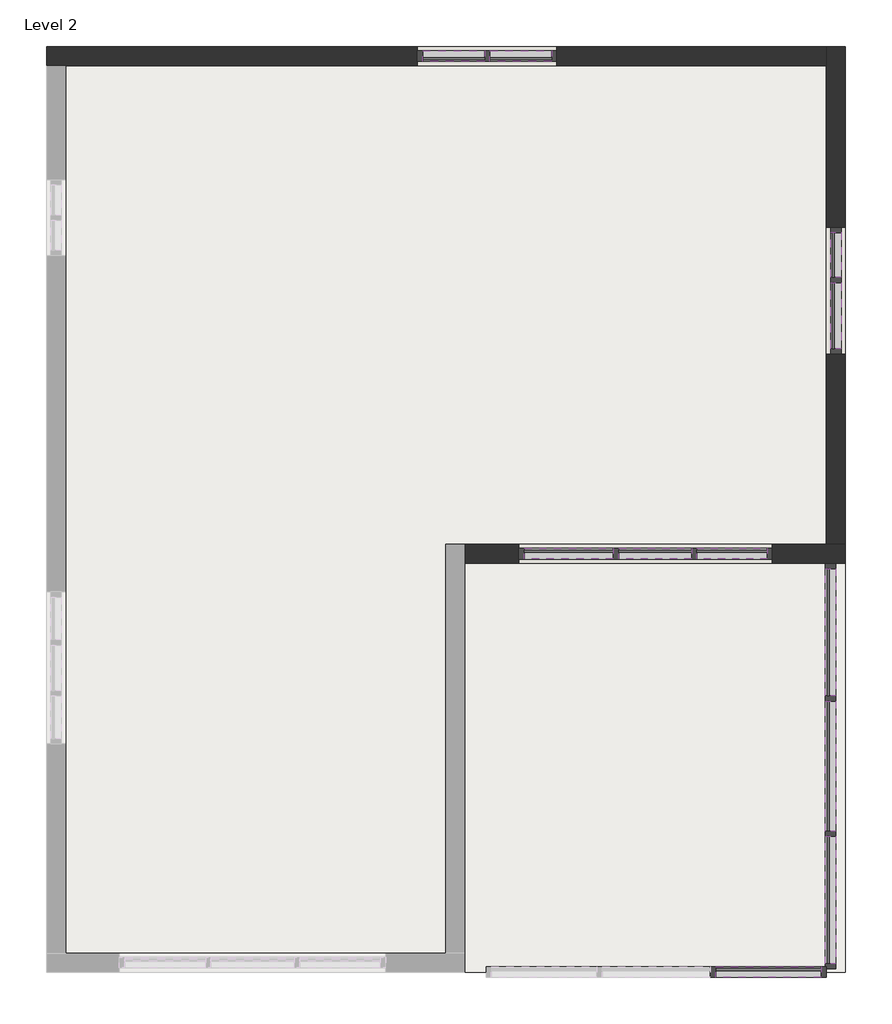
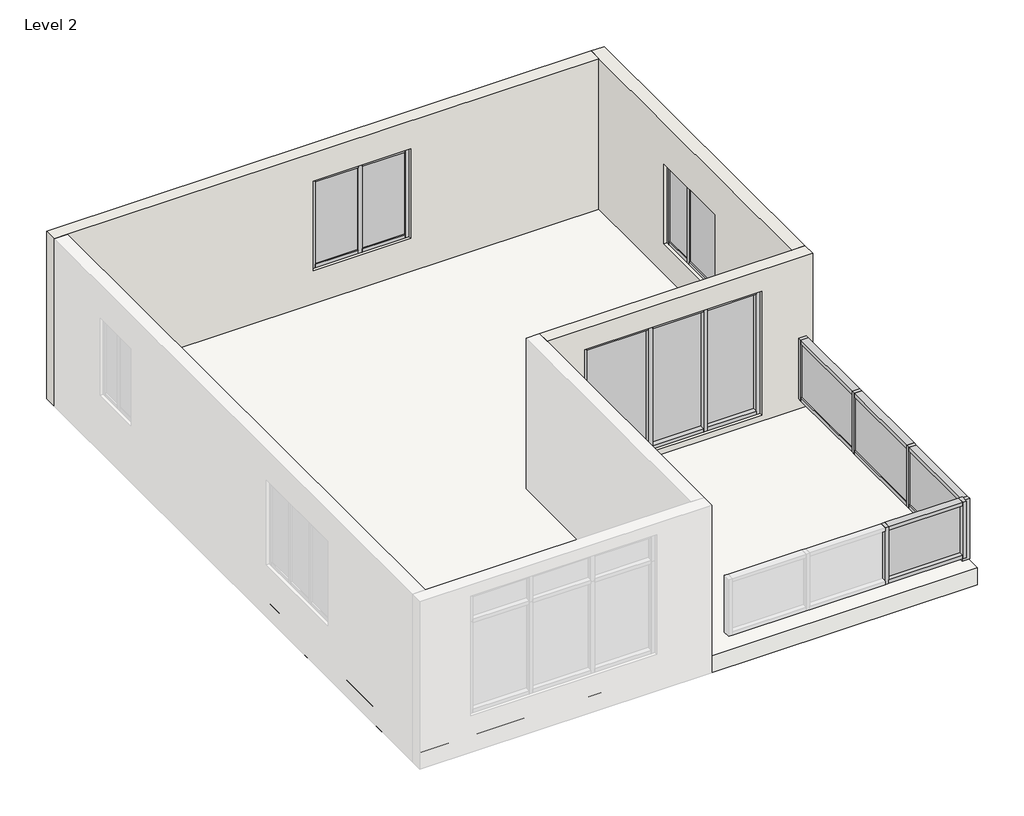
# One storey, part 2 of 2: 38 members, 11 plates, 3 walls, 1 roof.
"""IFC4 building model written with IfcOpenShell, lengths in millimetres."""

from ifc_helpers import new_model, si_unit, frame, origin, place, context, project, spatial, polyline, outline, extrude, faceted_brep, transform, mapped, element, save
from components import member_81de2198, member_99b0d556, member_4d6ef9b1, member_3974447c, member_c3d994c2, member_091e92f8, member_eb359e9e, member_20160837, member_02f15020, member_8e1b9e66, member_e29be78d, member_3eefc08a, member_e90b2f09, member_13dc6413, member_ee8fd4dd, member_c59792e9, member_3a0a7659, member_1a0dfb12, member_62f62403, system_panel_glazed_a9a9195b, system_panel_glazed_303585a9, system_panel_glazed_dbec328f, system_panel_glazed_6a79ef8b, system_panel_glazed_b7516aa2, system_panel_glazed_3160786d, system_panel_glazed_8fb7f6e3, system_panel_glazed_63ee4140, system_panel_glazed_1c093cbc

model = new_model("IFC4")

# Units and contexts
model_context = context("Model", 3, world=origin())
ifc_project = project(units=[si_unit("LENGTHUNIT", "METRE", prefix="MILLI")], contexts=[model_context])

# Site, building, storey
site = spatial("IfcSite", under=ifc_project)
building = spatial("IfcBuilding", under=site)
storey = spatial("IfcBuildingStorey", under=building, Name="Level 2", Elevation=3048.0)

# Members
placement = place(None, origin())
member_shape = member_81de2198(model_context)
element("IfcMember", 1, ObjectType="Rectangular Mullion : 2.5\" x 5\" rectangular", at=placement, inside=storey, context=model_context, shape_type="MappedRepresentation", body=[
    mapped(member_shape, transform((-8098.3518575, -6804.4878384, 3902.8712854), x_axis=(0.0, 0.0, -1.0), y_axis=(1.0, 0.0, 0.0), z_axis=(0.0, -1.0, 0.0))),
])
element("IfcMember", 2, ObjectType="Rectangular Mullion : 2.5\" x 5\" rectangular", at=placement, inside=storey, context=model_context, shape_type="MappedRepresentation", body=[
    mapped(member_shape, transform((-8098.3518575, -6264.7378384, 5354.7619868), x_axis=(0.0, 0.0, 1.0), y_axis=(1.0, 0.0, 0.0), z_axis=(0.0, 1.0, 0.0))),
])
member_2_shape = member_99b0d556(model_context)
element("IfcMember", 3, ObjectType="Rectangular Mullion : 2.5\" x 5\" rectangular", at=placement, inside=storey, context=model_context, shape_type="MappedRepresentation", body=[
    mapped(member_2_shape, transform((-10708.2018575, -10125.5378384, 3460.4214945), x_axis=(0.0, 0.0, -1.0), y_axis=(0.0, -1.0, 0.0), z_axis=(-1.0, 0.0, 0.0))),
])
member_3_shape = member_4d6ef9b1(model_context)
element("IfcMember", 4, ObjectType="Rectangular Mullion : 2.5\" x 5\" rectangular", at=placement, inside=storey, context=model_context, shape_type="MappedRepresentation", body=[
    mapped(member_3_shape, transform((-11844.8518575, -10125.5378384, 3460.4214945), x_axis=(0.0, 0.0, -1.0), y_axis=(0.0, -1.0, 0.0), z_axis=(-1.0, 0.0, 0.0))),
])
member_4_shape = member_3974447c(model_context)
element("IfcMember", 5, ObjectType="Rectangular Mullion : 2.5\" x 5\" rectangular", at=placement, inside=storey, context=model_context, shape_type="MappedRepresentation", body=[
    mapped(member_4_shape, transform((-9800.1518575, -10125.5378384, 3460.4214945), x_axis=(1.0, 0.0, 0.0), y_axis=(0.0, -1.0, 0.0), z_axis=(0.0, 0.0, -1.0))),
])
element("IfcMember", 6, ObjectType="Rectangular Mullion : 2.5\" x 5\" rectangular", at=placement, inside=storey, context=model_context, shape_type="MappedRepresentation", body=[
    mapped(member_4_shape, transform((-10739.9518575, -10125.5378384, 3460.4214945), x_axis=(1.0, 0.0, 0.0), y_axis=(0.0, -1.0, 0.0), z_axis=(0.0, 0.0, -1.0))),
])
element("IfcMember", 7, ObjectType="Rectangular Mullion : 2.5\" x 5\" rectangular", at=placement, inside=storey, context=model_context, shape_type="MappedRepresentation", body=[
    mapped(member_2_shape, transform((-9831.9018575, -10125.5378384, 5714.786093), x_axis=(0.0, 0.0, 1.0), y_axis=(0.0, -1.0, 0.0), z_axis=(1.0, 0.0, 0.0))),
])
element("IfcMember", 8, ObjectType="Rectangular Mullion : 2.5\" x 5\" rectangular", at=placement, inside=storey, context=model_context, shape_type="MappedRepresentation", body=[
    mapped(member_3_shape, transform((-10771.7018575, -10125.5378384, 5714.786093), x_axis=(0.0, 0.0, 1.0), y_axis=(0.0, -1.0, 0.0), z_axis=(1.0, 0.0, 0.0))),
])
member_5_shape = member_c3d994c2(model_context)
element("IfcMember", 9, ObjectType="Rectangular Mullion : 2.5\" x 5\" rectangular", at=placement, inside=storey, context=model_context, shape_type="MappedRepresentation", body=[
    mapped(member_5_shape, transform((-11908.3518575, -10125.5378384, 5714.786093), x_axis=(-1.0, 0.0, 0.0), y_axis=(0.0, -1.0, 0.0), z_axis=(0.0, 0.0, 1.0))),
])
member_6_shape = member_091e92f8(model_context)
element("IfcMember", 10, ObjectType="Rectangular Mullion : 2.5\" x 5\" rectangular", at=placement, inside=storey, context=model_context, shape_type="MappedRepresentation", body=[
    mapped(member_6_shape, transform((-9768.4018575, -10125.5378384, 3460.4214945), x_axis=(0.0, 0.0, -1.0), y_axis=(0.0, -1.0, 0.0), z_axis=(-1.0, 0.0, 0.0))),
])
element("IfcMember", 11, ObjectType="Rectangular Mullion : 2.5\" x 5\" rectangular", at=placement, inside=storey, context=model_context, shape_type="MappedRepresentation", body=[
    mapped(member_6_shape, transform((-8923.8518575, -10125.5378384, 5714.786093), x_axis=(0.0, 0.0, 1.0), y_axis=(0.0, -1.0, 0.0), z_axis=(1.0, 0.0, 0.0))),
])
element("IfcMember", 12, ObjectType="Rectangular Mullion : 2.5\" x 5\" rectangular", at=placement, inside=storey, context=model_context, shape_type="MappedRepresentation", body=[
    mapped(member_5_shape, transform((-8860.3518575, -10125.5378384, 3460.4214945), x_axis=(1.0, 0.0, 0.0), y_axis=(0.0, -1.0, 0.0), z_axis=(0.0, 0.0, -1.0))),
])
member_7_shape = member_eb359e9e(model_context)
element("IfcMember", 13, ObjectType="Rectangular Mullion : 2.5\" x 5\" rectangular", at=placement, inside=storey, context=model_context, shape_type="MappedRepresentation", body=[
    mapped(member_7_shape, transform((-8276.1518575, -15154.7378384, 4689.3272807), x_axis=(0.0, 0.0, 1.0), y_axis=(0.0, -1.0, 0.0), z_axis=(1.0, 0.0, 0.0))),
])
element("IfcMember", 14, ObjectType="Rectangular Mullion : 2.5\" x 5\" rectangular", at=placement, inside=storey, context=model_context, shape_type="MappedRepresentation", body=[
    mapped(member_7_shape, transform((-9544.0351909, -15154.7378384, 3657.6), x_axis=(0.0, 0.0, -1.0), y_axis=(0.0, -1.0, 0.0), z_axis=(-1.0, 0.0, 0.0))),
])
member_8_shape = member_20160837(model_context)
element("IfcMember", 15, ObjectType="Rectangular Mullion : 2.5\" x 5\" rectangular", at=placement, inside=storey, context=model_context, shape_type="MappedRepresentation", body=[
    mapped(member_8_shape, transform((-9575.7851909, -15154.7378384, 3657.6), x_axis=(1.0, 0.0, 0.0), y_axis=(0.0, -1.0, 0.0), z_axis=(0.0, 0.0, -1.0))),
])
member_9_shape = member_02f15020(model_context)
element("IfcMember", 16, ObjectType="Rectangular Mullion : 2.5\" x 5\" rectangular", at=placement, inside=storey, context=model_context, shape_type="MappedRepresentation", body=[
    mapped(member_9_shape, transform((-8212.6518575, -15154.7378384, 3657.6), x_axis=(1.0, 0.0, 0.0), y_axis=(0.0, -1.0, 0.0), z_axis=(0.0, 0.0, -1.0))),
])
member_10_shape = member_8e1b9e66(model_context)
element("IfcMember", 17, ObjectType="Rectangular Mullion : 2.5\" x 5\" rectangular", at=placement, inside=storey, context=model_context, shape_type="MappedRepresentation", body=[
    mapped(member_10_shape, transform((-8160.2387627, -13522.2465167, 4639.9432926), x_axis=(0.0, 0.0, 1.0), y_axis=(1.0, 0.0, 0.0), z_axis=(0.0, 1.0, 0.0))),
])
element("IfcMember", 18, ObjectType="Rectangular Mullion : 2.5\" x 5\" rectangular", at=placement, inside=storey, context=model_context, shape_type="MappedRepresentation", body=[
    mapped(member_10_shape, transform((-8160.2387627, -10303.3378384, 4639.9432926), x_axis=(0.0, 0.0, 1.0), y_axis=(1.0, 0.0, 0.0), z_axis=(0.0, 1.0, 0.0))),
])
member_11_shape = member_e29be78d(model_context)
element("IfcMember", 19, ObjectType="Rectangular Mullion : 2.5\" x 5\" rectangular", at=placement, inside=storey, context=model_context, shape_type="MappedRepresentation", body=[
    mapped(member_11_shape, transform((-8160.2387627, -11896.9171776, 4639.9432926), x_axis=(0.0, 0.0, 1.0), y_axis=(1.0, 0.0, 0.0), z_axis=(0.0, 1.0, 0.0))),
])
member_12_shape = member_3eefc08a(model_context)
element("IfcMember", 20, ObjectType="Rectangular Mullion : 2.5\" x 5\" rectangular", at=placement, inside=storey, context=model_context, shape_type="MappedRepresentation", body=[
    mapped(member_12_shape, transform((-8160.2387627, -13490.4965167, 3533.6625279), x_axis=(0.0, 1.0, 0.0), y_axis=(1.0, 0.0, 0.0), z_axis=(0.0, 0.0, -1.0))),
])
element("IfcMember", 21, ObjectType="Rectangular Mullion : 2.5\" x 5\" rectangular", at=placement, inside=storey, context=model_context, shape_type="MappedRepresentation", body=[
    mapped(member_12_shape, transform((-8160.2387627, -11865.1671776, 3533.6625279), x_axis=(0.0, 1.0, 0.0), y_axis=(1.0, 0.0, 0.0), z_axis=(0.0, 0.0, -1.0))),
])
element("IfcMember", 22, ObjectType="Rectangular Mullion : 2.5\" x 5\" rectangular", at=placement, inside=storey, context=model_context, shape_type="MappedRepresentation", body=[
    mapped(member_10_shape, transform((-8160.2387627, -11833.4171776, 3533.6625279), x_axis=(0.0, 0.0, -1.0), y_axis=(1.0, 0.0, 0.0), z_axis=(0.0, -1.0, 0.0))),
])
element("IfcMember", 23, ObjectType="Rectangular Mullion : 2.5\" x 5\" rectangular", at=placement, inside=storey, context=model_context, shape_type="MappedRepresentation", body=[
    mapped(member_10_shape, transform((-8160.2387627, -15052.3258559, 3533.6625279), x_axis=(0.0, 0.0, -1.0), y_axis=(1.0, 0.0, 0.0), z_axis=(0.0, -1.0, 0.0))),
])
element("IfcMember", 24, ObjectType="Rectangular Mullion : 2.5\" x 5\" rectangular", at=placement, inside=storey, context=model_context, shape_type="MappedRepresentation", body=[
    mapped(member_11_shape, transform((-8160.2387627, -13458.7465167, 3533.6625279), x_axis=(0.0, 0.0, -1.0), y_axis=(1.0, 0.0, 0.0), z_axis=(0.0, -1.0, 0.0))),
])
member_13_shape = member_e90b2f09(model_context)
element("IfcMember", 25, ObjectType="Rectangular Mullion : 2.5\" x 5\" rectangular", at=placement, inside=storey, context=model_context, shape_type="MappedRepresentation", body=[
    mapped(member_13_shape, transform((-8160.2387627, -15115.8258559, 4639.9432926), x_axis=(0.0, -1.0, 0.0), y_axis=(1.0, 0.0, 0.0), z_axis=(0.0, 0.0, 1.0))),
])
element("IfcMember", 26, ObjectType="Rectangular Mullion : 2.5\" x 5\" rectangular", at=placement, inside=storey, context=model_context, shape_type="MappedRepresentation", body=[
    mapped(member_13_shape, transform((-8160.2387627, -10239.8378384, 3533.6625279), x_axis=(0.0, 1.0, 0.0), y_axis=(1.0, 0.0, 0.0), z_axis=(0.0, 0.0, -1.0))),
])
member_14_shape = member_13dc6413(model_context)
element("IfcMember", 27, ObjectType="Rectangular Mullion : 2.5\" x 5\" rectangular", at=placement, inside=storey, context=model_context, shape_type="MappedRepresentation", body=[
    mapped(member_14_shape, transform((-8098.3518575, -6867.9878384, 5354.7619868), x_axis=(0.0, 0.0, 1.0), y_axis=(1.0, 0.0, 0.0), z_axis=(0.0, 1.0, 0.0))),
])
member_15_shape = member_ee8fd4dd(model_context)
element("IfcMember", 28, ObjectType="Rectangular Mullion : 2.5\" x 5\" rectangular", at=placement, inside=storey, context=model_context, shape_type="MappedRepresentation", body=[
    mapped(member_15_shape, transform((-8098.3518575, -6836.2378384, 3902.8712854), x_axis=(0.0, 1.0, 0.0), y_axis=(1.0, 0.0, 0.0), z_axis=(0.0, 0.0, -1.0))),
])
element("IfcMember", 29, ObjectType="Rectangular Mullion : 2.5\" x 5\" rectangular", at=placement, inside=storey, context=model_context, shape_type="MappedRepresentation", body=[
    mapped(member_14_shape, transform((-8098.3518575, -7661.7378384, 3902.8712854), x_axis=(0.0, 0.0, -1.0), y_axis=(1.0, 0.0, 0.0), z_axis=(0.0, -1.0, 0.0))),
])
member_16_shape = member_c59792e9(model_context)
element("IfcMember", 30, ObjectType="Rectangular Mullion : 2.5\" x 5\" rectangular", at=placement, inside=storey, context=model_context, shape_type="MappedRepresentation", body=[
    mapped(member_16_shape, transform((-8098.3518575, -6201.2378384, 3902.8712854), x_axis=(0.0, 1.0, 0.0), y_axis=(1.0, 0.0, 0.0), z_axis=(0.0, 0.0, -1.0))),
])
element("IfcMember", 31, ObjectType="Rectangular Mullion : 2.5\" x 5\" rectangular", at=placement, inside=storey, context=model_context, shape_type="MappedRepresentation", body=[
    mapped(member_16_shape, transform((-8098.3518575, -7725.2378384, 5354.7619868), x_axis=(0.0, -1.0, 0.0), y_axis=(1.0, 0.0, 0.0), z_axis=(0.0, 0.0, 1.0))),
])
member_17_shape = member_3a0a7659(model_context)
element("IfcMember", 32, ObjectType="Rectangular Mullion : 2.5\" x 5\" rectangular", at=placement, inside=storey, context=model_context, shape_type="MappedRepresentation", body=[
    mapped(member_17_shape, transform((-12257.6018575, -4143.8378384, 5584.2385429), x_axis=(0.0, 0.0, 1.0), y_axis=(0.0, 1.0, 0.0), z_axis=(-1.0, 0.0, 0.0))),
])
element("IfcMember", 33, ObjectType="Rectangular Mullion : 2.5\" x 5\" rectangular", at=placement, inside=storey, context=model_context, shape_type="MappedRepresentation", body=[
    mapped(member_17_shape, transform((-13064.0518575, -4143.8378384, 5584.2385429), x_axis=(0.0, 0.0, 1.0), y_axis=(0.0, 1.0, 0.0), z_axis=(-1.0, 0.0, 0.0))),
])
member_18_shape = member_1a0dfb12(model_context)
element("IfcMember", 34, ObjectType="Rectangular Mullion : 2.5\" x 5\" rectangular", at=placement, inside=storey, context=model_context, shape_type="MappedRepresentation", body=[
    mapped(member_18_shape, transform((-12289.3518575, -4143.8378384, 3955.4729812), x_axis=(-1.0, 0.0, 0.0), y_axis=(0.0, 1.0, 0.0), z_axis=(0.0, 0.0, -1.0))),
])
element("IfcMember", 35, ObjectType="Rectangular Mullion : 2.5\" x 5\" rectangular", at=placement, inside=storey, context=model_context, shape_type="MappedRepresentation", body=[
    mapped(member_17_shape, transform((-12321.1018575, -4143.8378384, 3955.4729812), x_axis=(0.0, 0.0, -1.0), y_axis=(0.0, 1.0, 0.0), z_axis=(1.0, 0.0, 0.0))),
])
element("IfcMember", 36, ObjectType="Rectangular Mullion : 2.5\" x 5\" rectangular", at=placement, inside=storey, context=model_context, shape_type="MappedRepresentation", body=[
    mapped(member_17_shape, transform((-11514.6518575, -4143.8378384, 3955.4729812), x_axis=(0.0, 0.0, -1.0), y_axis=(0.0, 1.0, 0.0), z_axis=(1.0, 0.0, 0.0))),
])
member_19_shape = member_62f62403(model_context)
element("IfcMember", 37, ObjectType="Rectangular Mullion : 2.5\" x 5\" rectangular", at=placement, inside=storey, context=model_context, shape_type="MappedRepresentation", body=[
    mapped(member_19_shape, transform((-13127.5518575, -4143.8378384, 3955.4729812), x_axis=(-1.0, 0.0, 0.0), y_axis=(0.0, 1.0, 0.0), z_axis=(0.0, 0.0, -1.0))),
])
element("IfcMember", 38, ObjectType="Rectangular Mullion : 2.5\" x 5\" rectangular", at=placement, inside=storey, context=model_context, shape_type="MappedRepresentation", body=[
    mapped(member_19_shape, transform((-11451.1518575, -4143.8378384, 5584.2385429), x_axis=(1.0, 0.0, 0.0), y_axis=(0.0, 1.0, 0.0), z_axis=(0.0, 0.0, 1.0))),
])

# Plates
system_panel_glazed_shape = system_panel_glazed_a9a9195b(model_context)
element("IfcPlate", 39, ObjectType="System Panel : Glazed", at=placement, inside=storey, context=model_context, shape_type="MappedRepresentation", body=[
    mapped(system_panel_glazed_shape, transform((-11308.2768575, -10125.5378384, 3523.9214945), x_axis=(1.0, 0.0, 0.0), y_axis=(0.0, 1.0, 0.0), z_axis=(0.0, 0.0, 1.0))),
])
system_panel_glazed_2_shape = system_panel_glazed_303585a9(model_context)
element("IfcPlate", 40, ObjectType="System Panel : Glazed", at=placement, inside=storey, context=model_context, shape_type="MappedRepresentation", body=[
    mapped(system_panel_glazed_2_shape, transform((-10270.0518575, -10125.5378384, 3523.9214945), x_axis=(1.0, 0.0, 0.0), y_axis=(0.0, 1.0, 0.0), z_axis=(0.0, 0.0, 1.0))),
])
system_panel_glazed_3_shape = system_panel_glazed_dbec328f(model_context)
element("IfcPlate", 41, ObjectType="System Panel : Glazed", at=placement, inside=storey, context=model_context, shape_type="MappedRepresentation", body=[
    mapped(system_panel_glazed_3_shape, transform((-9346.1268575, -10125.5378384, 3523.9214945), x_axis=(1.0, 0.0, 0.0), y_axis=(0.0, 1.0, 0.0), z_axis=(0.0, 0.0, 1.0))),
])
system_panel_glazed_4_shape = system_panel_glazed_6a79ef8b(model_context)
element("IfcPlate", 42, ObjectType="System Panel : Glazed", at=placement, inside=storey, context=model_context, shape_type="MappedRepresentation", body=[
    mapped(system_panel_glazed_4_shape, transform((-8910.0935242, -15154.7378384, 3721.1), x_axis=(1.0, 0.0, 0.0), y_axis=(0.0, 1.0, 0.0), z_axis=(0.0, 0.0, 1.0))),
])
system_panel_glazed_5_shape = system_panel_glazed_b7516aa2(model_context)
element("IfcPlate", 43, ObjectType="System Panel : Glazed", at=placement, inside=storey, context=model_context, shape_type="MappedRepresentation", body=[
    mapped(system_panel_glazed_5_shape, transform((-8160.2387627, -14287.2861863, 3597.1625279), x_axis=(0.0, 1.0, 0.0), y_axis=(-1.0, 0.0, 0.0), z_axis=(0.0, 0.0, 1.0))),
])
element("IfcPlate", 44, ObjectType="System Panel : Glazed", at=placement, inside=storey, context=model_context, shape_type="MappedRepresentation", body=[
    mapped(system_panel_glazed_5_shape, transform((-8160.2387627, -11068.377508, 3597.1625279), x_axis=(0.0, 1.0, 0.0), y_axis=(-1.0, 0.0, 0.0), z_axis=(0.0, 0.0, 1.0))),
])
system_panel_glazed_6_shape = system_panel_glazed_3160786d(model_context)
element("IfcPlate", 45, ObjectType="System Panel : Glazed", at=placement, inside=storey, context=model_context, shape_type="MappedRepresentation", body=[
    mapped(system_panel_glazed_6_shape, transform((-8160.2387627, -12677.8318471, 3597.1625279), x_axis=(0.0, 1.0, 0.0), y_axis=(-1.0, 0.0, 0.0), z_axis=(0.0, 0.0, 1.0))),
])
system_panel_glazed_7_shape = system_panel_glazed_8fb7f6e3(model_context)
element("IfcPlate", 46, ObjectType="System Panel : Glazed", at=placement, inside=storey, context=model_context, shape_type="MappedRepresentation", body=[
    mapped(system_panel_glazed_7_shape, transform((-8098.3518575, -7264.8628384, 3966.3712854), x_axis=(0.0, 1.0, 0.0), y_axis=(-1.0, 0.0, 0.0), z_axis=(0.0, 0.0, 1.0))),
])
system_panel_glazed_8_shape = system_panel_glazed_63ee4140(model_context)
element("IfcPlate", 47, ObjectType="System Panel : Glazed", at=placement, inside=storey, context=model_context, shape_type="MappedRepresentation", body=[
    mapped(system_panel_glazed_8_shape, transform((-8098.3518575, -6534.6128384, 3966.3712854), x_axis=(0.0, 1.0, 0.0), y_axis=(-1.0, 0.0, 0.0), z_axis=(0.0, 0.0, 1.0))),
])
system_panel_glazed_9_shape = system_panel_glazed_1c093cbc(model_context)
element("IfcPlate", 48, ObjectType="System Panel : Glazed", at=placement, inside=storey, context=model_context, shape_type="MappedRepresentation", body=[
    mapped(system_panel_glazed_9_shape, transform((-11886.1268575, -4143.8378384, 4018.9729812), x_axis=(-1.0, 0.0, 0.0), y_axis=(0.0, -1.0, 0.0), z_axis=(0.0, 0.0, 1.0))),
])
element("IfcPlate", 49, ObjectType="System Panel : Glazed", at=placement, inside=storey, context=model_context, shape_type="MappedRepresentation", body=[
    mapped(system_panel_glazed_9_shape, transform((-12692.5768575, -4143.8378384, 4018.9729812), x_axis=(-1.0, 0.0, 0.0), y_axis=(0.0, -1.0, 0.0), z_axis=(0.0, 0.0, 1.0))),
])

# Roof
element("IfcRoof", 50, ObjectType="Generic - 12\"", at=placement, inside=storey, context=model_context, shape_type="SweptSolid", body=[
    extrude(outline(polyline([(-17585.2518575, -4029.5378384), (-7984.0518575, -4029.5378384), (-7984.0518575, -15154.7378384), (-17585.2518575, -15154.7378384), (-17585.2518575, -4029.5378384)])), frame((0.0, 0.0, 3048.0), z_axis=(0.0, 0.0, 1.0), x_axis=(1.0, 0.0, 0.0)), (0.0, 0.0, 1.0), 304.8),
])

# Walls
element("IfcWall", 51, ObjectType="9\"", at=placement, inside=storey, context=model_context, shape_type="Brep", body=[
    faceted_brep([(-12556.0518575, -10239.8378384, 3048.0), (-7984.0518575, -10239.8378384, 3048.0), (-7984.0518575, -10239.8378384, 6096.0), (-12556.0518575, -10239.8378384, 6096.0), (-11908.3518575, -10239.8378384, 3460.4214945), (-11908.3518575, -10239.8378384, 5714.786093), (-8860.3518575, -10239.8378384, 5714.786093), (-8860.3518575, -10239.8378384, 3460.4214945), (-7984.0518575, -10011.2378384, 3048.0), (-8212.6518575, -10011.2378384, 3048.0), (-12556.0518575, -10011.2378384, 3048.0), (-12556.0518575, -10011.2378384, 6096.0), (-8212.6518575, -10011.2378384, 6096.0), (-7984.0518575, -10011.2378384, 6096.0), (-11908.3518575, -10011.2378384, 5714.786093), (-11908.3518575, -10011.2378384, 3460.4214945), (-8860.3518575, -10011.2378384, 3460.4214945), (-8860.3518575, -10011.2378384, 5714.786093)], [[[0, 1, 2, 3], [4, 5, 6, 7]], [[8, 9, 10, 11, 12, 13], [14, 15, 16, 17]], [[1, 0, 10, 9, 8]], [[3, 2, 13, 12, 11]], [[0, 3, 11, 10]], [[2, 1, 8, 13]], [[4, 15, 14, 5]], [[5, 14, 17, 6]], [[6, 17, 16, 7]], [[15, 4, 7, 16]]]),
])
element("IfcWall", 52, ObjectType="9\"", at=placement, inside=storey, context=model_context, shape_type="Brep", body=[
    faceted_brep([(-7984.0518575, -10011.2378384, 3048.0), (-7984.0518575, -4029.5378384, 3048.0), (-7984.0518575, -4029.5378384, 6096.0), (-7984.0518575, -10011.2378384, 6096.0), (-7984.0518575, -7725.2378384, 3902.8712854), (-7984.0518575, -7725.2378384, 5354.7619868), (-7984.0518575, -6201.2378384, 5354.7619868), (-7984.0518575, -6201.2378384, 3902.8712854), (-8212.6518575, -4029.5378384, 3048.0), (-8212.6518575, -4258.1378384, 3048.0), (-8212.6518575, -10011.2378384, 3048.0), (-8212.6518575, -10011.2378384, 6096.0), (-8212.6518575, -4258.1378384, 6096.0), (-8212.6518575, -4029.5378384, 6096.0), (-8212.6518575, -7725.2378384, 5354.7619868), (-8212.6518575, -7725.2378384, 3902.8712854), (-8212.6518575, -6201.2378384, 3902.8712854), (-8212.6518575, -6201.2378384, 5354.7619868)], [[[0, 1, 2, 3], [4, 5, 6, 7]], [[8, 9, 10, 11, 12, 13], [14, 15, 16, 17]], [[1, 0, 10, 9, 8]], [[3, 2, 13, 12, 11]], [[0, 3, 11, 10]], [[2, 1, 8, 13]], [[4, 15, 14, 5]], [[5, 14, 17, 6]], [[6, 17, 16, 7]], [[15, 4, 7, 16]]]),
])
element("IfcWall", 53, ObjectType="9\"", at=placement, inside=storey, context=model_context, shape_type="Brep", body=[
    faceted_brep([(-8212.6518575, -4029.5378384, 3048.0), (-17585.2518575, -4029.5378384, 3048.0), (-17585.2518575, -4029.5378384, 6096.0), (-8212.6518575, -4029.5378384, 6096.0), (-11451.1518575, -4029.5378384, 3955.4729812), (-11451.1518575, -4029.5378384, 5584.2385429), (-13127.5518575, -4029.5378384, 5584.2385429), (-13127.5518575, -4029.5378384, 3955.4729812), (-17585.2518575, -4258.1378384, 3048.0), (-17356.6518575, -4258.1378384, 3048.0), (-8212.6518575, -4258.1378384, 3048.0), (-8212.6518575, -4258.1378384, 6096.0), (-17356.6518575, -4258.1378384, 6096.0), (-17585.2518575, -4258.1378384, 6096.0), (-11451.1518575, -4258.1378384, 5584.2385429), (-11451.1518575, -4258.1378384, 3955.4729812), (-13127.5518575, -4258.1378384, 3955.4729812), (-13127.5518575, -4258.1378384, 5584.2385429)], [[[0, 1, 2, 3], [4, 5, 6, 7]], [[8, 9, 10, 11, 12, 13], [14, 15, 16, 17]], [[1, 0, 10, 9, 8]], [[3, 2, 13, 12, 11]], [[0, 3, 11, 10]], [[2, 1, 8, 13]], [[4, 15, 14, 5]], [[5, 14, 17, 6]], [[6, 17, 16, 7]], [[15, 4, 7, 16]]]),
])

save(model, "model.ifc")

# Revit data of these elements
# Type "Rectangular Mullion : 2.5\" x 5\" rectangular"
#   built-in parameter 1007304 = 0.416667 (stored number, unit not read)
#   built-in parameter 1007301 = 0.104167 (stored number, unit not read)
#   built-in parameter 1007300 = 0.104167 (stored number, unit not read)
# Type "System Panel : Glazed"
#   Construction Type Id = "GSP4R"
#   Analytic Construction = "1/8 in Pilkington single glazing"
#   Visual Light Transmittance = 0.9
#   Solar Heat Gain Coefficient = 0.86
#   Heat Transfer Coefficient (U) = 1.18115 BTU/(h·ft²·°F)
#   Define Thermal Properties by = 1
# Type "Generic - 12\""
#   Assembly Code = "B1020"
#   Layers, outside or top first: 1' - 0" no material (function 1)
# Type "9\""
#   Assembly Code = "B2010"
#   Layers, outside or top first: 0' - 9" no material (function 1)
# Elements 1, 2, 3, 4, 5, 6, 7, 8, 9, 10, 11, 12, 13, 14, 15, 16, 17, 18, 19, 20, 21, 22, 23, 24, 25, 26, 27, 28, 29, 30, 31, 32, 33, 34, 35, 36, 37, 38 (IfcMember, "Rectangular Mullion : 2.5\" x 5\" rectangular")
#   Phase Created = New Construction
#   Materials on its faces: "Aluminum"
# Elements 39, 40, 41, 42, 43, 44, 45, 46, 47, 48, 49 (IfcPlate, "System Panel : Glazed")
#   Phase Created = New Construction
#   Materials on its faces: "Glass"
# Element 50 (IfcRoof, "Generic - 12\"")
#   built-in parameter 1001705 = 11 (stored number, unit not read)
#   built-in parameter 1001710 = 33615
#   Phase Created = New Construction
#   Materials on its faces: "Default Roof"
# Elements 51, 52, 53 (IfcWall, "9\"")
#   Top Offset = 0' - 0"
#   Base Offset = 0' - 0"
#   Unconnected Height = 10' - 0"
#   wall height = 10' - 0"
#   Phase Created = New Construction
#   Base Constraint = Level 2
#   Materials on its faces: "Default Wall"
# Materials
#   "Aluminum": class "Metal", colour RGB 247 247 247, transparency 0, Description = "Aluminum 6061", Cost = 0
#   "Glass": class "Glass", colour RGB 0 128 192, transparency 0.75, Description = "Soda Lime Glass", Cost = 0
#   "Default Roof": colour RGB 88 101 114, transparency 0, Cost = 0
#   "Default Wall": colour RGB 128 128 128, transparency 0, Cost = 0
